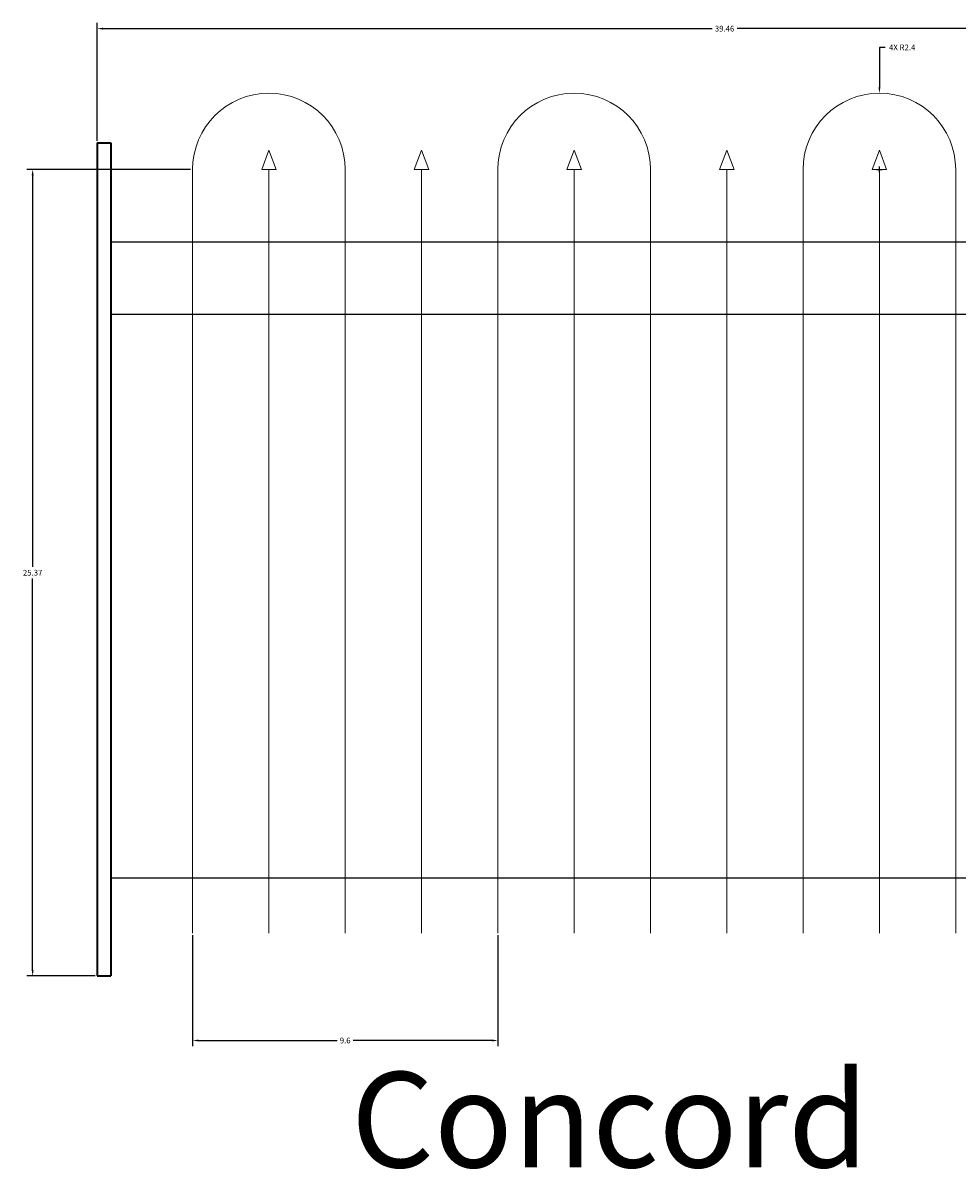
# Model space of a CAD drawing. Units: inches. Extents: x 756 to 915, y 488 to 695.
# Tile 13 of 25: x 815 to 844, y 588 to 624. Entities that reach past the tile are written whole.
import ezdxf

# ---------------------------------------------------------------- set-up
doc = ezdxf.new("R2010")
doc.units = ezdxf.units.IN
doc.header["$MEASUREMENT"] = 0
for name, color, linetype, lineweight in [('L-ANNO-TEXT', 7, 'Continuous', 25), ('L-FENC-PCKT', 7, 'Continuous', 18), ('L-FENC-POST', 7, 'Continuous', 35), ('L-FENC-RAIL', 7, 'Continuous', 25), ('M-DIMS', 2, 'Continuous', 18)]:
    doc.layers.add(name, color=color, linetype=linetype, lineweight=lineweight)
doc.styles.get("Standard").update_dxf_attribs({"font": 'arial.ttf'})
doc.dimstyles.get("Standard").update_dxf_attribs({"dimtxt": 0.18, "dimasz": 0.18, "dimexe": 0.18, "dimexo": 0.0625, "dimgap": 0.09, "dimtad": 0, "dimtih": 1, "dimtoh": 1, "dimdec": 0, "dimzin": 0, "dimdsep": 46, "dimlunit": 3, "dimtxsty": 'Standard', "dimcen": 0.09, "dimadec": 0, "dimazin": 0, "dimtfac": 1, "dimtdec": 0, "dimtofl": 0, "dimtmove": 0, "dimatfit": 3, "dimfxl": 1, "dimtolj": 1, "dimtzin": 0, "dimarcsym": 0})

# ---------------------------------------------------------------- blocks, each defined once
blk = doc.blocks.new('FENCE-POST-LEFT')
for p, q in [((0, 26.207), (0, 0)), ((0, 26.207), (0.426, 26.207)), ((0.426, 26.207), (0.426, 0)), ((0.426, 26.207), (0.426, 0)), ((0, 0), (0.426, 0))]:
    blk.add_line(p, q)
blk = doc.blocks.new('PICKET-ROUND-ARCH')
for p, q in [((0, 24.019), (0, 0)), ((4.8, 24.019), (4.8, 0))]:
    blk.add_line(p, q)
blk.add_arc((2.4, 24.019), 2.4, 0, 180)
blk = doc.blocks.new('PICKET-SPEAR-ARCH-INFILL')
blk.add_line((0.227, 24.019), (0.227, 0))
blk.add_lwpolyline([(0.227, 24.019), (0, 24.019), (0.227, 24.631), (0.455, 24.019)], close=True)
blk = doc.blocks.new('*D53')
at = {"layer": 'Defpoints', "color": 0, "transparency": 16777216}
for p in [(856.791, 623.683), (817.332, 620.092), (856.791, 620.092)]:
    blk.add_point(p, dxfattribs=at)
at = {"layer": 'M-DIMS', "color": 0, "lineweight": -2, "transparency": 16777216}
for p, q in [((817.332, 620.154), (817.332, 623.863)), ((856.791, 620.154), (856.791, 623.863)), ((817.512, 623.683), (836.668, 623.683)), ((856.611, 623.683), (837.455, 623.683))]:
    blk.add_line(p, q, dxfattribs=at)
at = {"layer": 'M-DIMS', "color": 0, "transparency": 16777216}
for points in [[(817.512, 623.713), (817.512, 623.653), (817.332, 623.683)], [(856.611, 623.713), (856.611, 623.653), (856.791, 623.683)]]:
    blk.add_solid(points, dxfattribs=at)
at = {"layer": 'M-DIMS', "color": 0, "transparency": 16777216, "insert": (837.062, 623.683), "char_height": 0.18, "attachment_point": 5}
blk.add_mtext('\\A1;39.46', dxfattribs=at)
blk = doc.blocks.new('*D55')
at = {"layer": 'Defpoints', "color": 0, "transparency": 16777216}
for p in [(815.302, 619.253), (820.332, 619.253), (817.332, 593.885)]:
    blk.add_point(p, dxfattribs=at)
at = {"layer": 'M-DIMS', "color": 0, "lineweight": -2, "transparency": 16777216}
for p, q in [((820.269, 619.253), (815.122, 619.253)), ((815.302, 619.073), (815.302, 606.751)), ((815.302, 594.065), (815.302, 606.387)), ((817.27, 593.885), (815.122, 593.885))]:
    blk.add_line(p, q, dxfattribs=at)
at = {"layer": 'M-DIMS', "color": 0, "transparency": 16777216}
for points in [[(815.272, 619.073), (815.332, 619.073), (815.302, 619.253)], [(815.272, 594.065), (815.332, 594.065), (815.302, 593.885)]]:
    blk.add_solid(points, dxfattribs=at)
at = {"layer": 'M-DIMS', "color": 0, "transparency": 16777216, "insert": (815.302, 606.569), "char_height": 0.18, "attachment_point": 5}
blk.add_mtext('\\A1;25.37', dxfattribs=at)
blk = doc.blocks.new('*D57')
at = {"layer": 'Defpoints', "color": 0, "transparency": 16777216}
for p in [(820.332, 595.234), (829.931, 595.234), (829.931, 591.855)]:
    blk.add_point(p, dxfattribs=at)
at = {"layer": 'M-DIMS', "color": 0, "lineweight": -2, "transparency": 16777216}
for p, q in [((820.332, 595.172), (820.332, 591.675)), ((829.931, 595.172), (829.931, 591.675)), ((820.512, 591.855), (824.878, 591.855)), ((829.751, 591.855), (825.385, 591.855))]:
    blk.add_line(p, q, dxfattribs=at)
at = {"layer": 'M-DIMS', "color": 0, "transparency": 16777216}
for points in [[(820.512, 591.885), (820.512, 591.825), (820.332, 591.855)], [(829.751, 591.885), (829.751, 591.825), (829.931, 591.855)]]:
    blk.add_solid(points, dxfattribs=at)
at = {"layer": 'M-DIMS', "color": 0, "transparency": 16777216, "insert": (825.131, 591.855), "char_height": 0.18, "attachment_point": 5}
blk.add_mtext('\\A1;9.6', dxfattribs=at)
blk = doc.blocks.new('*D80')
at = {"layer": 'Defpoints', "color": 0, "transparency": 16777216}
for p in [(841.931, 621.653), (841.931, 619.253)]:
    blk.add_point(p, dxfattribs=at)
at = {"layer": 'M-DIMS', "color": 0, "lineweight": -2, "transparency": 16777216}
for p, q in [((842.111, 623.093), (841.931, 623.093)), ((841.931, 623.093), (841.931, 621.833)), ((841.841, 619.253), (842.021, 619.253)), ((841.931, 619.163), (841.931, 619.343))]:
    blk.add_line(p, q, dxfattribs=at)
at = {"layer": 'M-DIMS', "color": 0, "transparency": 16777216}
blk.add_solid([(841.901, 621.833), (841.961, 621.833), (841.931, 621.653)], dxfattribs=at)
at = {"layer": 'M-DIMS', "color": 0, "transparency": 16777216, "insert": (842.648, 623.093), "char_height": 0.18, "attachment_point": 5}
blk.add_mtext('\\A1;4X R2.4', dxfattribs=at)

msp = doc.modelspace()

# ---------------------------------------------------------------- linework, layer by layer
at = {"layer": 'L-FENC-RAIL'}
for p, q in [((817.7591, 616.9765), (856.3639, 616.9765)), ((817.7591, 614.7001), (856.3639, 614.7001)), ((817.7591, 596.9663), (856.3639, 596.9663))]:
    msp.add_line(p, q, dxfattribs=at)

# ---------------------------------------------------------------- block references
at = {"layer": 'L-FENC-PCKT'}
for name, p in [('PICKET-ROUND-ARCH', (820.3311, 595.234)), ('PICKET-ROUND-ARCH', (829.9307, 595.234)), ('PICKET-ROUND-ARCH', (839.5304, 595.234)), ('PICKET-SPEAR-ARCH-INFILL', (822.5041, 595.234)), ('PICKET-SPEAR-ARCH-INFILL', (827.3039, 595.234)), ('PICKET-SPEAR-ARCH-INFILL', (832.1037, 595.234)), ('PICKET-SPEAR-ARCH-INFILL', (836.9035, 595.234)), ('PICKET-SPEAR-ARCH-INFILL', (841.7034, 595.234))]:
    msp.add_blockref(name, p, dxfattribs=at)
at = {"layer": 'L-FENC-POST'}
msp.add_blockref('FENCE-POST-LEFT', (817.3328, 593.8847), dxfattribs=at)

# ---------------------------------------------------------------- texts
at = {"layer": 'L-ANNO-TEXT'}
msp.add_text('Concord', height=3, dxfattribs=at).set_placement((825.3134, 587.8635))

# ---------------------------------------------------------------- dimensions: what is measured, and where the dimension line sits
at = {"layer": 'M-DIMS'}
for base, p1, p2, override, picture, middle in [((856.7906, 623.6829), (817.3324, 620.0915), (856.7906, 620.0915), {"dimdec": 2, "dimlfac": 1, "dimrnd": 0, "dimzin": 0, "dimdsep": 46, "dimlunit": 2}, '*D53', (837.0615, 623.6829)), ((829.9312, 591.8547), (820.3316, 595.2343), (829.9312, 595.2343), {"dimdec": 1, "dimlfac": 1, "dimrnd": 0, "dimzin": 0, "dimdsep": 46, "dimlunit": 2}, '*D57', (825.1314, 591.8547))]:
    dim = msp.add_linear_dim(base=base, p1=p1, p2=p2, dimstyle='Standard', override=override, dxfattribs=at)
    dim.commit()
    dim.dimension.update_dxf_attribs({"geometry": picture, "text_midpoint": middle})
dim = msp.add_radius_dim(center=(841.9308, 619.2529), mpoint=(841.931, 621.6529), text='4X <>', dimstyle='Standard', override={"dimdec": 1, "dimlfac": 1, "dimrnd": 0, "dimzin": 0, "dimdsep": 46, "dimlunit": 2}, dxfattribs=at)
dim.commit()
dim.dimension.update_dxf_attribs({"geometry": '*D80', "text_midpoint": (842.6478, 623.0928), "dimtype": 164})
dim = msp.add_linear_dim(base=(815.3024, 619.2529), p1=(817.3324, 593.8847), p2=(820.3316, 619.2529), angle=90, dimstyle='Standard', override={"dimdec": 2, "dimlfac": 1, "dimrnd": 0, "dimzin": 0, "dimdsep": 46, "dimlunit": 2}, dxfattribs=at)
dim.commit()
dim.dimension.update_dxf_attribs({"geometry": '*D55', "text_midpoint": (815.3024, 606.5688)})

doc.saveas('drawing.dxf')
